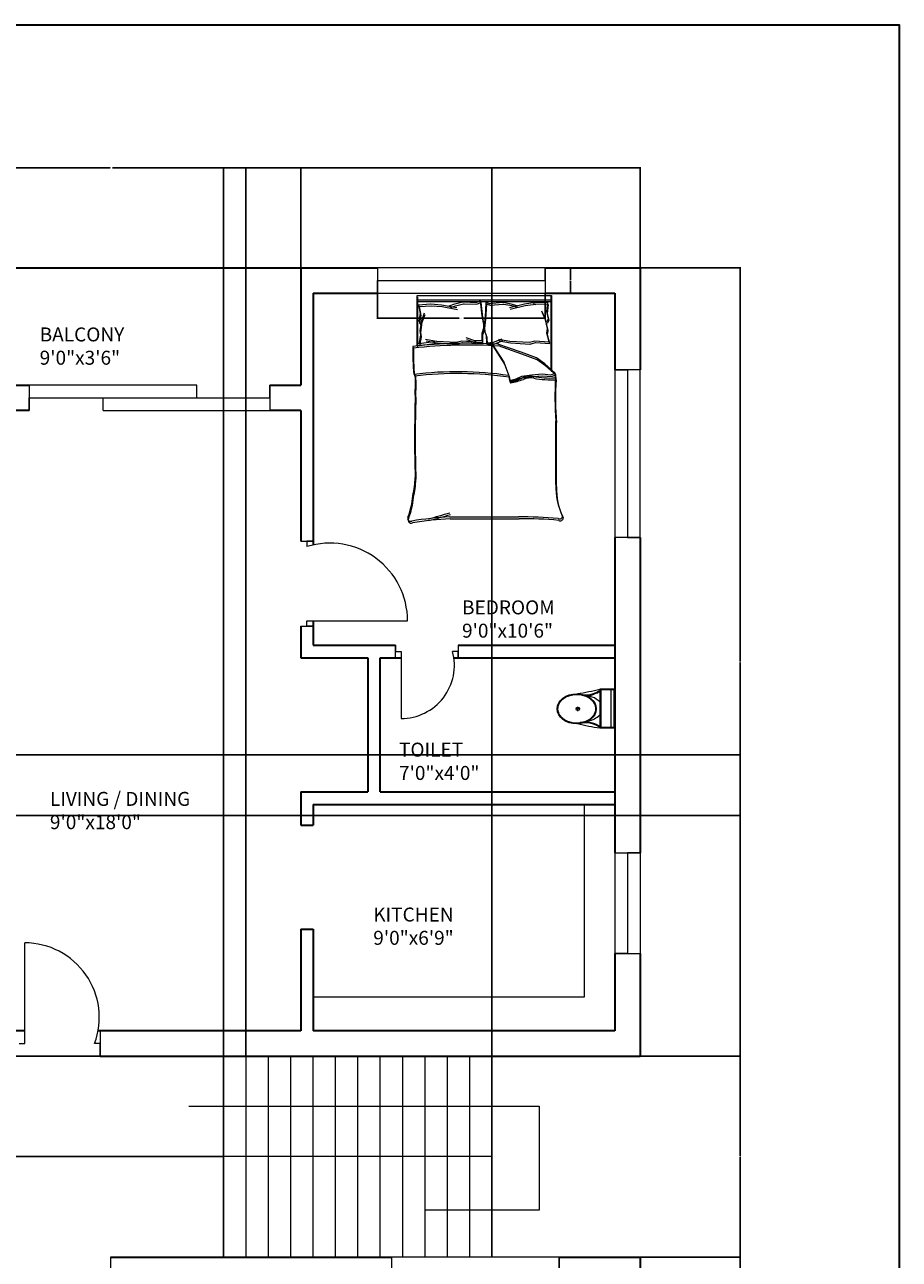
# Model space of a CAD drawing. Units: inches. Extents: x 2527 to 3140, y 1564 to 2435.
# Tile 4 of 4: x 2827 to 3140, y 1993 to 2435. Entities that reach past the tile are written whole.
import ezdxf

# ---------------------------------------------------------------- set-up
doc = ezdxf.new("R2010")
doc.units = ezdxf.units.IN
for name, color, linetype, lineweight in [('A-ANNO-DIMS', 2, 'Continuous', 18), ('A-ANNO-TTLB', 7, 'Continuous', 35), ('A-AREA-IDEN', 7, 'Continuous', 18), ('A-DOOR', 191, 'Continuous', 18), ('A-FLOR-CASE', 9, 'Continuous', 18), ('A-FLOR-FIXT', 7, 'Continuous', 18), ('A-FLOR-STRS', 81, 'Continuous', 18), ('A-FURN', 8, 'Continuous', 13), ('A-GLAZ', 131, 'Continuous', 18), ('A-WALL', 7, 'Continuous', 35)]:
    doc.layers.add(name, color=color, linetype=linetype, lineweight=lineweight)
doc.styles.get("Standard").update_dxf_attribs({"font": 'arial.ttf'})
doc.dimstyles.get("Standard").update_dxf_attribs({"dimtxt": 0.18, "dimasz": 0.18, "dimexe": 0.18, "dimexo": 0.0625, "dimgap": 0.09, "dimtad": 0, "dimtih": 1, "dimtoh": 1, "dimdec": 4, "dimzin": 0, "dimdsep": 46, "dimtxsty": 'Standard', "dimcen": 0.09, "dimadec": 0, "dimazin": 0, "dimtfac": 1, "dimtdec": 4, "dimtofl": 0, "dimtmove": 0, "dimatfit": 3, "dimfxl": 1, "dimtolj": 1, "dimtzin": 0, "dimarcsym": 0})

# ---------------------------------------------------------------- blocks, each defined once
blk = doc.blocks.new('A$C31115884')
for p, q in [((283, 498), (223, 498)), ((258, 466), (258, 523)), ((0, 200), (0, 0)), ((520, 200), (0, 200)), ((10, 190), (10, 10)), ((510, 190), (10, 190)), ((510, 10), (510, 190)), ((520, 0), (520, 200)), ((510, 54), (0, 54)), ((10, 10), (510, 10)), ((0, 0), (520, 0))]:
    blk.add_line(p, q)
blk.add_circle((256, 496), 23.6)
for centre, radius, start, end in [((2778, -205), 2807, 165.4549, 171.7133), ((3237, 905), 2807, 188.2867, 194.5451), ((-295, 403), 365, 324.2091, 9.3499), ((-295, 403), 375, 324.2091, 9.3499), ((384, 406), 293, 190.2774, 224.1564), ((139, 406), 293, 315.8436, 2.6563), ((806, 403), 375, 179.2036, 215.7909), ((806, 403), 365, 170.6501, 215.7909)]:
    blk.add_arc(centre, radius, start, end)
blk.add_ellipse((256, 510), major_axis=(0, -261), ratio=0.772727)
blk.add_open_spline([(256, 259), (263, 259), (270, 260), (288, 262), (299, 265), (320, 273), (330, 278), (350, 291), (360, 299), (378, 316), (386, 326), (402, 347), (409, 358), (421, 383), (427, 395), (436, 422), (440, 436), (445, 465), (447, 480), (448, 509), (448, 524), (445, 553), (443, 568), (436, 596), (432, 610), (422, 636), (416, 649), (402, 672), (395, 683), (379, 703), (370, 712), (351, 728), (341, 735), (321, 746), (310, 751), (289, 757), (278, 759), (256, 761), (245, 761), (223, 757), (212, 754), (191, 746), (181, 741), (161, 728), (151, 720), (133, 703), (125, 693), (110, 672), (103, 660), (90, 636), (85, 623), (76, 596), (72, 582), (67, 553), (66, 538), (64, 509), (65, 494), (68, 465), (70, 450), (77, 422), (81, 408), (91, 382), (97, 370), (111, 346), (118, 335), (135, 316), (144, 307), (162, 291), (172, 284), (193, 273), (203, 269), (225, 262), (236, 260), (250, 259), (253, 259), (256, 259)], degree=3, knots=[0, 0, 0, 0, 0.110105, 0.110105, 0.285049, 0.285049, 0.459994, 0.459994, 0.634938, 0.634938, 0.809882, 0.809882, 0.984827, 0.984827, 1.159771, 1.159771, 1.334715, 1.334715, 1.50966, 1.50966, 1.684604, 1.684604, 1.859549, 1.859549, 2.034493, 2.034493, 2.209437, 2.209437, 2.384382, 2.384382, 2.559326, 2.559326, 2.73427, 2.73427, 2.909215, 2.909215, 3.084159, 3.084159, 3.259103, 3.259103, 3.434048, 3.434048, 3.608992, 3.608992, 3.783936, 3.783936, 3.958881, 3.958881, 4.133825, 4.133825, 4.30877, 4.30877, 4.483714, 4.483714, 4.658658, 4.658658, 4.833603, 4.833603, 5.008547, 5.008547, 5.183491, 5.183491, 5.358436, 5.358436, 5.53338, 5.53338, 5.708324, 5.708324, 5.883269, 5.883269, 6.058213, 6.058213, 6.233158, 6.233158, 6.283185, 6.283185, 6.283185, 6.283185])
blk = doc.blocks.new('BED-DOUBLE')
for p, q in [((3.48, 63.33), (3.48, 81.44)), ((3.48, 63.33), (3.48, 81.44)), ((3.48, 81.44), (51.49, 81.44)), ((3.48, 79.91), (51.27, 79.91)), ((3.48, 79.91), (51.27, 79.91)), ((3.7, 62.69), (3.7, 80.8)), ((3.7, 62.69), (3.7, 80.8)), ((24.54, 78.99), (25.98, 79.57)), ((24.54, 78.99), (25.98, 79.57)), ((25.98, 79.57), (26.56, 74.22)), ((25.98, 79.57), (26.56, 74.22)), ((51.27, 81.44), (51.27, 54.83)), ((51.27, 81.44), (51.27, 54.83)), ((51.49, 81.44), (51.49, 80.8)), ((51.49, 80.8), (51.49, 54.19)), ((51.49, 80.8), (51.49, 54.19)), ((3.7, 79.27), (51.49, 79.27)), ((3.7, 79.27), (51.49, 79.27)), ((3.89, 78.13), (4.47, 74.95)), ((3.9, 78.1), (8.18, 78.43)), ((3.9, 78.1), (8.18, 78.43)), ((3.9, 78.13), (4.47, 74.95)), ((4.12, 77.49), (4.7, 74.31)), ((4.12, 77.49), (4.7, 74.31)), ((4.13, 77.47), (8.41, 77.79)), ((4.13, 77.47), (8.41, 77.79)), ((5.05, 72.49), (6.06, 75.24)), ((5.05, 72.49), (6.06, 75.24)), ((8.18, 78.43), (8.29, 78.42)), ((8.18, 78.43), (8.29, 78.42)), ((8.29, 78.42), (12.11, 78.13)), ((8.29, 78.42), (12.11, 78.13)), ((8.41, 77.79), (8.51, 77.78)), ((8.41, 77.79), (8.51, 77.78)), ((8.51, 77.78), (12.34, 77.49)), ((8.51, 77.78), (12.34, 77.49)), ((12.11, 78.13), (17.6, 77.11)), ((12.11, 78.13), (17.6, 77.11)), ((12.34, 77.49), (17.83, 76.48)), ((12.34, 77.49), (17.83, 76.48)), ((14.86, 77.69), (16.88, 78.42)), ((14.86, 77.69), (16.88, 78.42)), ((15.08, 77.05), (17.11, 77.78)), ((15.08, 77.05), (17.11, 77.78)), ((16.88, 78.42), (19.77, 79.14)), ((16.88, 78.42), (19.77, 79.14)), ((17.11, 77.78), (20, 78.5)), ((17.11, 77.78), (20, 78.5)), ((19.77, 79.14), (20.09, 79.14)), ((19.77, 79.14), (20.09, 79.14)), ((20, 78.5), (20.32, 78.5)), ((20, 78.5), (20.32, 78.5)), ((20.09, 79.14), (24.54, 78.99)), ((20.09, 79.14), (24.54, 78.99)), ((20.32, 78.5), (24.77, 78.35)), ((20.32, 78.5), (24.77, 78.35)), ((24.77, 78.35), (26.21, 78.93)), ((24.77, 78.35), (26.21, 78.93)), ((26.21, 78.93), (26.79, 73.58)), ((26.21, 78.93), (26.79, 73.58)), ((27.98, 78.95), (27.73, 73.58)), ((27.98, 78.95), (27.73, 73.58)), ((28.21, 78.31), (27.96, 72.94)), ((28.21, 78.31), (27.96, 72.94)), ((29.46, 78.46), (27.98, 78.95)), ((29.46, 78.46), (27.98, 78.95)), ((29.68, 77.82), (28.21, 78.31)), ((29.68, 77.82), (28.21, 78.31)), ((33.88, 78.89), (29.46, 78.46)), ((33.88, 78.89), (29.46, 78.46)), ((34.11, 78.25), (29.68, 77.82)), ((34.11, 78.25), (29.68, 77.82)), ((34.21, 78.91), (33.88, 78.89)), ((34.2, 78.91), (33.88, 78.89)), ((34.43, 78.27), (34.11, 78.25)), ((34.43, 78.27), (34.11, 78.25)), ((37.14, 78.36), (34.2, 78.91)), ((37.14, 78.36), (34.21, 78.91)), ((37.36, 77.73), (34.43, 78.27)), ((37.36, 77.73), (34.43, 78.27)), ((41.91, 78.37), (36.5, 77.02)), ((41.91, 78.37), (36.5, 77.02)), ((42.14, 77.73), (36.72, 76.38)), ((42.14, 77.73), (36.72, 76.38)), ((39.2, 77.77), (37.14, 78.36)), ((39.2, 77.77), (37.14, 78.36)), ((39.43, 77.13), (37.36, 77.73)), ((39.43, 77.13), (37.36, 77.73)), ((45.71, 78.9), (41.91, 78.37)), ((45.71, 78.9), (41.91, 78.37)), ((45.94, 78.26), (42.14, 77.73)), ((45.94, 78.26), (42.14, 77.73)), ((50.11, 78.89), (44.71, 78.98)), ((44.71, 78.98), (45.71, 78.9)), ((50.11, 78.89), (44.71, 78.98)), ((44.71, 78.98), (45.71, 78.9)), ((50.34, 78.25), (44.94, 78.34)), ((44.94, 78.34), (45.94, 78.26)), ((50.34, 78.25), (44.94, 78.34)), ((44.94, 78.34), (45.94, 78.26)), ((49.31, 73.19), (48.13, 75.86)), ((49.31, 73.19), (48.13, 75.86)), ((49.54, 72.55), (48.36, 75.23)), ((49.54, 72.55), (48.36, 75.23)), ((50.11, 78.89), (49.73, 75.68)), ((50.11, 78.89), (49.73, 75.68)), ((49.73, 75.68), (50.33, 73.1)), ((49.73, 75.68), (50.33, 73.1)), ((50.34, 78.25), (49.96, 75.04)), ((50.34, 78.25), (49.96, 75.04)), ((4.47, 74.95), (4.04, 72.34)), ((4.47, 74.95), (4.04, 72.34)), ((4.04, 72.34), (4.62, 71.33)), ((4.04, 72.34), (4.62, 71.33)), ((4.7, 74.31), (4.27, 71.7)), ((4.7, 74.31), (4.27, 71.7)), ((4.27, 71.7), (4.85, 70.69)), ((4.27, 71.7), (4.85, 70.69)), ((4.47, 68.87), (5.05, 72.49)), ((4.47, 68.87), (5.05, 72.49)), ((4.7, 68.23), (5.28, 71.85)), ((4.7, 68.23), (5.28, 71.85)), ((5.28, 71.85), (6.29, 74.6)), ((5.28, 71.85), (6.29, 74.6)), ((26.56, 74.22), (27.14, 71.04)), ((26.56, 74.22), (27.14, 71.04)), ((26.79, 73.58), (27.37, 70.4)), ((26.79, 73.58), (27.37, 70.4)), ((27.14, 71.04), (27.14, 69.74)), ((27.14, 71.04), (27.14, 69.74)), ((27.73, 73.58), (27.36, 70.36)), ((27.73, 73.58), (27.36, 70.36)), ((27.96, 72.94), (27.58, 69.73)), ((27.96, 72.94), (27.58, 69.73)), ((50.11, 69.61), (49.31, 73.19)), ((50.11, 69.61), (49.31, 73.19)), ((50.34, 68.97), (49.54, 72.55)), ((50.34, 68.97), (49.54, 72.55)), ((50.33, 73.1), (49.81, 72.06)), ((50.33, 73.1), (49.82, 72.06)), ((49.96, 75.04), (50.56, 72.47)), ((49.96, 75.04), (50.56, 72.47)), ((50.56, 72.47), (50.04, 71.42)), ((50.56, 72.47), (50.04, 71.42)), ((4.18, 64.1), (4.76, 67.28)), ((4.18, 64.1), (4.76, 67.28)), ((4.41, 63.46), (4.99, 66.64)), ((4.41, 63.46), (4.99, 66.64)), ((4.76, 67.28), (4.47, 68.87)), ((4.76, 67.28), (4.47, 68.87)), ((4.99, 66.64), (4.7, 68.23)), ((4.99, 66.64), (4.7, 68.23)), ((24.1, 65.18), (20.96, 66.27)), ((24.1, 65.18), (20.96, 66.27)), ((27.14, 69.74), (26.56, 67.86)), ((27.14, 69.74), (26.56, 67.86)), ((26.56, 67.86), (26.56, 65.18)), ((26.56, 67.86), (26.56, 65.18)), ((27.37, 69.1), (26.79, 67.22)), ((27.37, 69.1), (26.79, 67.22)), ((26.79, 67.22), (26.79, 64.54)), ((26.79, 67.22), (26.79, 64.54)), ((27.36, 70.36), (27.44, 69.07)), ((27.36, 70.36), (27.44, 69.07)), ((27.37, 70.4), (27.37, 69.1)), ((27.37, 70.4), (27.37, 69.1)), ((27.44, 69.07), (28.13, 67.23)), ((27.44, 69.07), (28.13, 67.23)), ((27.58, 69.73), (27.66, 68.43)), ((27.58, 69.73), (27.66, 68.43)), ((27.66, 68.43), (28.36, 66.59)), ((27.66, 68.43), (28.36, 66.59)), ((28.13, 67.23), (28.3, 64.55)), ((28.13, 67.23), (28.3, 64.55)), ((28.36, 66.59), (28.53, 63.91)), ((28.36, 66.59), (28.53, 63.91)), ((49.92, 68.01), (50.11, 69.61)), ((49.92, 68.01), (50.11, 69.61)), ((50.7, 64.87), (49.92, 68.01)), ((50.7, 64.87), (49.92, 68.01)), ((50.15, 67.37), (50.34, 68.97)), ((50.15, 67.37), (50.34, 68.97)), ((50.93, 64.23), (50.15, 67.37)), ((50.93, 64.23), (50.15, 67.37)), ((9.28, 64.82), (4.18, 64.1)), ((9.28, 64.82), (4.18, 64.1)), ((9.51, 64.19), (4.41, 63.46)), ((9.51, 64.19), (4.41, 63.46)), ((6.38, 65.81), (10.41, 65.15)), ((6.38, 65.81), (10.41, 65.15)), ((6.61, 65.17), (10.64, 64.51)), ((6.61, 65.17), (10.64, 64.51)), ((10.41, 65.15), (9.28, 64.82)), ((10.41, 65.15), (9.28, 64.82)), ((10.64, 64.51), (9.51, 64.19)), ((10.64, 64.51), (9.51, 64.19)), ((10.41, 65.15), (17.42, 64.72)), ((10.41, 65.15), (17.42, 64.72)), ((10.64, 64.51), (17.65, 64.08)), ((10.64, 64.51), (17.65, 64.08)), ((17.42, 64.72), (19.38, 65.27)), ((17.42, 64.72), (19.38, 65.27)), ((17.65, 64.08), (19.61, 64.63)), ((17.65, 64.08), (19.61, 64.63)), ((19.38, 65.27), (24.52, 64.87)), ((19.38, 65.27), (24.52, 64.87)), ((19.61, 64.63), (24.74, 64.23)), ((19.61, 64.63), (24.74, 64.23)), ((24.33, 64.54), (21.19, 65.63)), ((24.33, 64.54), (21.19, 65.63)), ((26.56, 65.18), (24.1, 65.18)), ((26.56, 65.18), (24.1, 65.18)), ((26.79, 64.54), (24.33, 64.54)), ((26.79, 64.54), (24.33, 64.54)), ((28.3, 64.55), (30.75, 64.7)), ((28.3, 64.55), (30.75, 64.7)), ((28.53, 63.91), (30.98, 64.06)), ((28.53, 63.91), (30.98, 64.06)), ((30.26, 64.06), (34.45, 57.57)), ((30.26, 64.06), (34.45, 57.57)), ((30.49, 63.42), (34.68, 56.93)), ((30.49, 63.42), (34.68, 56.93)), ((30.75, 64.7), (33.82, 65.99)), ((30.75, 64.7), (33.82, 65.99)), ((30.98, 64.06), (34.05, 65.35)), ((30.98, 64.06), (34.05, 65.35)), ((40.64, 61.13), (32.31, 64.06)), ((40.64, 61.13), (32.31, 64.06)), ((40.87, 60.49), (32.53, 63.42)), ((40.87, 60.49), (32.54, 63.42)), ((32.56, 65.81), (36.6, 65.15)), ((32.56, 65.81), (36.6, 65.15)), ((32.79, 65.17), (36.83, 64.51)), ((32.79, 65.17), (36.82, 64.51)), ((36.6, 65.15), (43.61, 64.72)), ((36.6, 65.15), (43.61, 64.72)), ((36.82, 64.51), (43.83, 64.08)), ((36.83, 64.51), (43.84, 64.08)), ((43.61, 64.72), (45.57, 65.27)), ((43.61, 64.72), (45.57, 65.27)), ((43.83, 64.08), (45.8, 64.63)), ((43.84, 64.08), (45.8, 64.63)), ((45.57, 65.27), (50.7, 64.87)), ((45.57, 65.27), (50.7, 64.87)), ((45.8, 64.63), (50.93, 64.23)), ((45.8, 64.63), (50.93, 64.23)), ((34.45, 57.57), (36.15, 53.08)), ((34.45, 57.57), (36.15, 53.08)), ((46.22, 59.11), (40.64, 61.13)), ((46.22, 59.11), (40.64, 61.13)), ((46.45, 58.47), (40.87, 60.49)), ((46.45, 58.47), (40.87, 60.49)), ((49.16, 56.95), (46.22, 59.11)), ((49.16, 56.95), (46.22, 59.11)), ((49.39, 56.31), (46.45, 58.47)), ((49.39, 56.31), (46.45, 58.47)), ((34.68, 56.93), (36.38, 52.44)), ((34.68, 56.93), (36.38, 52.44)), ((36.15, 53.08), (36.46, 51.07)), ((36.15, 53.08), (36.46, 51.07)), ((40.95, 52.61), (44.36, 53.08)), ((40.95, 52.61), (44.36, 53.08)), ((44.36, 53.08), (48.23, 53.39)), ((44.36, 53.08), (48.23, 53.39)), ((48.23, 53.39), (51.33, 53.08)), ((48.23, 53.39), (51.33, 53.08)), ((52.87, 53.7), (49.16, 56.95)), ((52.87, 53.7), (49.16, 56.95)), ((53.1, 53.06), (49.39, 56.31)), ((53.1, 53.06), (49.39, 56.31)), ((51.33, 53.08), (52.87, 53.7)), ((51.33, 53.08), (52.87, 53.7)), ((51.56, 52.44), (53.1, 53.06)), ((51.56, 52.44), (53.1, 53.06)), ((52.95, 51.95), (52.87, 53.7, 3.87)), ((52.95, 51.95), (52.87, 53.7, 3.87)), ((53.18, 51.31), (53.1, 53.06, 3.87)), ((53.18, 51.31), (53.1, 53.06, 3.87)), ((36.38, 52.44), (36.69, 50.43)), ((36.38, 52.44), (36.69, 50.43)), ((36.46, 51.07), (38.94, 51.68)), ((36.46, 51.07), (38.94, 51.68)), ((36.69, 50.43), (39.17, 51.05)), ((36.69, 50.43), (39.17, 51.05)), ((38.94, 51.68), (40.95, 52.61)), ((38.94, 51.68), (40.95, 52.61)), ((39.17, 51.05), (41.18, 51.97)), ((39.17, 51.05), (41.18, 51.97)), ((41.18, 51.97), (44.59, 52.44)), ((41.18, 51.97), (44.59, 52.44)), ((44.59, 52.44), (48.46, 52.75)), ((44.59, 52.44), (48.46, 52.75)), ((48.46, 52.75), (51.56, 52.44)), ((48.46, 52.75), (51.56, 52.44)), ((15.06, 2.2), (39.68, 2.2)), ((15.06, 2.2), (39.68, 2.2)), ((15.29, 1.56), (39.91, 1.56)), ((15.29, 1.56), (39.91, 1.56))]:
    blk.add_line(p, q)
for centre, radius, start, end in [((85.16, 61.35), 83.31, 178.7218, 185.604), ((85.16, 61.35), 83.31, 178.7218, 185.604), ((21.36, -100.61), 164.97, 86.0865, 96.7821), ((21.36, -100.61), 164.97, 86.0865, 96.7821), ((85.39, 60.71), 83.31, 178.7218, 185.604), ((85.39, 60.71), 83.31, 178.7218, 185.604), ((21.59, -101.25), 164.97, 86.0865, 96.7821), ((21.59, -101.25), 164.97, 86.0865, 96.7821), ((17.76, -74.87), 129.02, 81.7845, 96.9006), ((17.76, -74.87), 129.02, 81.7845, 96.9006), ((17.98, -75.51), 129.02, 81.7845, 96.9006), ((17.98, -75.51), 129.02, 81.7845, 96.9006), ((-167.31, 50.27), 170.11, 358.4762, 1.0082), ((-167.31, 50.27), 170.11, 358.4762, 1.0082), ((-167.08, 49.63), 170.11, 358.4762, 1.0082), ((-167.08, 49.63), 170.11, 358.4762, 1.0082), ((36.64, 51), 0.185, 160.2464, 271.1377), ((36.64, 51), 0.185, 160.2464, 271.1377), ((31.15, 79.96), 29.65, 280.6617, 289.8806), ((31.15, 79.96), 29.65, 280.6617, 289.8806), ((36.87, 50.36), 0.185, 160.2464, 271.1377), ((36.86, 50.36), 0.185, 160.2464, 271.1377), ((31.38, 79.32), 29.65, 280.6617, 289.8806), ((31.38, 79.32), 29.65, 280.6617, 289.8806), ((43.74, 46.38), 6.22, 78.6608, 113.7384), ((43.74, 46.38), 6.22, 78.6608, 113.7384), ((43.97, 45.74), 6.22, 78.6608, 113.7384), ((43.97, 45.74), 6.22, 78.6608, 113.7384), ((51.33, 88.1), 36.18, 259.8763, 272.5657), ((51.33, 88.1), 36.18, 259.8763, 272.5657), ((51.56, 87.46), 36.18, 259.8763, 272.5657), ((51.56, 87.46), 36.18, 259.8763, 272.5657), ((182.27, 45.13), 129.5, 176.9791, 183.8365), ((182.27, 45.13), 129.5, 176.9791, 183.8365), ((182.49, 44.49), 129.5, 176.9791, 183.8365), ((182.49, 44.49), 129.5, 176.9791, 183.8365), ((484.82, 30.83), 482.31, 178.2277, 181.7185), ((484.82, 30.83), 482.31, 178.2277, 181.7185), ((485.05, 30.19), 482.31, 178.2277, 181.7185), ((485.05, 30.19), 482.31, 178.2277, 181.7185), ((-4508.74, 13.62), 4561.86, 0.00217, 0.28689), ((-4508.74, 13.62), 4561.86, 0.00217, 0.28689), ((-4508.51, 12.98), 4561.86, 0.00217, 0.28689), ((-4508.51, 12.98), 4561.86, 0.00217, 0.28689), ((-26.9, 16.93), 29.63, 346.0648, 358.9113), ((-26.9, 16.93), 29.63, 346.0648, 358.9113), ((-26.67, 16.29), 29.63, 346.0648, 358.9113), ((-26.67, 16.29), 29.63, 346.0648, 358.9113), ((76.16, 12.78), 23.07, 177.4714, 206.4681), ((76.16, 12.78), 23.07, 177.4714, 206.4681), ((-21.66, 11.17), 23.56, 337.9751, 356.652), ((-21.66, 11.17), 23.56, 337.9751, 356.652), ((-21.43, 10.53), 23.56, 337.9751, 356.652), ((-21.43, 10.53), 23.56, 337.9751, 356.652), ((76.39, 12.14), 23.07, 177.4714, 206.4681), ((76.39, 12.14), 23.07, 177.4714, 206.4681), ((1.09, 1.73), 1.09, 146.1736, 293.4781), ((1.09, 1.73), 1.09, 146.1736, 293.4781), ((1.32, 1.09), 1.09, 146.1736, 293.4781), ((1.32, 1.09), 1.09, 146.1736, 293.4781), ((21.43, -119.39), 121.76, 92.9958, 99.4091), ((21.43, -119.39), 121.76, 92.9958, 99.4091), ((21.66, -120.03), 121.76, 92.9958, 99.4091), ((21.66, -120.03), 121.76, 92.9958, 99.4091), ((-17.22, 105.15), 106.46, 283.3832, 287.7053), ((-17.22, 105.15), 106.46, 283.3832, 287.7053), ((-16.99, 104.52), 106.46, 283.3832, 287.7053), ((-16.99, 104.52), 106.46, 283.3832, 287.7053), ((41.15, -130.83), 133.04, 84.4998, 90.6351), ((41.15, -130.83), 133.04, 84.4998, 90.6351), ((41.38, -131.47), 133.04, 84.4998, 90.6351), ((41.38, -131.47), 133.04, 84.4998, 90.6351), ((54.41, 2.57), 1.1, 242.6588, 356.02), ((54.41, 2.57), 1.1, 242.6588, 356.02), ((54.64, 1.93), 1.1, 242.6588, 356.02), ((54.64, 1.93), 1.1, 242.6588, 356.02)]:
    blk.add_arc(centre, radius, start, end)
blk = doc.blocks.new('WIN-60')
for p, q in [((0, 9), (0, 0)), ((60, 9), (0, 9)), ((60, 4.5), (60, 9)), ((60, 9), (60, 0)), ((0, 0), (0, 4.5)), ((0, 4.5), (60, 4.5)), ((0, 0), (60, 0))]:
    blk.add_line(p, q)
blk = doc.blocks.new('WIN-36')
for p, q in [((0, 36), (9, 36)), ((0, 36), (0, 0)), ((9, 36), (4.5, 36)), ((4.5, 36), (4.5, 0)), ((9, 36), (9, 0)), ((4.5, 0), (0, 0)), ((0, 0), (9, 0))]:
    blk.add_line(p, q)
blk = doc.blocks.new('*D7')
at = {"layer": 'A-ANNO-DIMS', "color": 0, "lineweight": -2, "transparency": 16777216}
for p, q in [((2953.62, 2339.08), (2953.62, 2329.96)), ((3013.62, 2339.08), (3013.62, 2329.96)), ((2953.8, 2330.14), (2982.77, 2330.14)), ((3013.44, 2330.14), (2984.46, 2330.14))]:
    blk.add_line(p, q, dxfattribs=at)
at = {"layer": 'A-ANNO-DIMS', "color": 0, "transparency": 16777216}
for points in [[(2953.8, 2330.17), (2953.8, 2330.11), (2953.62, 2330.14)], [(3013.44, 2330.17), (3013.44, 2330.11), (3013.62, 2330.14)]]:
    blk.add_solid(points, dxfattribs=at)
at = {"layer": 'Defpoints', "color": 0, "transparency": 16777216}
for p in [(2953.62, 2339.14), (3013.62, 2339.14), (3013.62, 2330.14)]:
    blk.add_point(p, dxfattribs=at)
at = {"layer": 'A-ANNO-DIMS', "color": 0, "transparency": 16777216, "insert": (2983.62, 2330.14), "char_height": 0.18, "attachment_point": 5}
blk.add_mtext('\\A1;WIN. 60 TYP.', dxfattribs=at)
blk = doc.blocks.new('*D8')
at = {"layer": 'A-ANNO-DIMS', "color": 0, "lineweight": -2, "transparency": 16777216}
for p, q in [((3013.68, 2348.14), (3022.8, 2348.14)), ((3022.62, 2347.96), (3022.62, 2343.82)), ((3022.62, 2339.32), (3022.62, 2343.46)), ((3013.68, 2339.14), (3022.8, 2339.14))]:
    blk.add_line(p, q, dxfattribs=at)
at = {"layer": 'A-ANNO-DIMS', "color": 0, "transparency": 16777216}
for points in [[(3022.59, 2347.96), (3022.65, 2347.96), (3022.62, 2348.14)], [(3022.59, 2339.32), (3022.65, 2339.32), (3022.62, 2339.14)]]:
    blk.add_solid(points, dxfattribs=at)
at = {"layer": 'Defpoints', "color": 0, "transparency": 16777216}
for p in [(3013.62, 2348.14), (3022.62, 2348.14), (3013.62, 2339.14)]:
    blk.add_point(p, dxfattribs=at)
at = {"layer": 'A-ANNO-DIMS', "color": 0, "transparency": 16777216, "insert": (3022.62, 2343.64), "char_height": 0.18, "attachment_point": 5}
blk.add_mtext('\\A1;9 TYP.', dxfattribs=at)
blk = doc.blocks.new('*D22')
at = {"layer": 'A-ANNO-DIMS', "color": 0, "lineweight": -2, "transparency": 16777216}
for p, q in [((2926.08, 2348.21), (2926.08, 2384.17)), ((2926.26, 2383.99), (2986.44, 2383.99)), ((3047.4, 2383.99), (2987.22, 2383.99)), ((3047.58, 2348.21), (3047.58, 2384.17))]:
    blk.add_line(p, q, dxfattribs=at)
at = {"layer": 'A-ANNO-DIMS', "color": 0, "transparency": 16777216}
for points in [[(2926.26, 2384.02), (2926.26, 2383.96), (2926.08, 2383.99)], [(3047.4, 2384.02), (3047.4, 2383.96), (3047.58, 2383.99)]]:
    blk.add_solid(points, dxfattribs=at)
at = {"layer": 'Defpoints', "color": 0, "transparency": 16777216}
for p in [(3047.58, 2383.99), (2926.08, 2348.14), (3047.58, 2348.14)]:
    blk.add_point(p, dxfattribs=at)
at = {"layer": 'A-ANNO-DIMS', "color": 0, "transparency": 16777216, "insert": (2986.83, 2383.99), "char_height": 0.18, "attachment_point": 5}
blk.add_mtext('\\A1;121.5', dxfattribs=at)
blk = doc.blocks.new('*D23')
at = {"layer": 'A-ANNO-DIMS', "color": 0, "lineweight": -2, "transparency": 16777216}
for p, q in [((3047.64, 1994.14), (3083.61, 1994.14)), ((3083.43, 1993.96), (3083.43, 1850.32)), ((3083.43, 1706.32), (3083.43, 1849.96)), ((3047.64, 1706.14), (3083.61, 1706.14))]:
    blk.add_line(p, q, dxfattribs=at)
at = {"layer": 'A-ANNO-DIMS', "color": 0, "transparency": 16777216}
for points in [[(3083.4, 1993.96), (3083.46, 1993.96), (3083.43, 1994.14)], [(3083.4, 1706.32), (3083.46, 1706.32), (3083.43, 1706.14)]]:
    blk.add_solid(points, dxfattribs=at)
at = {"layer": 'Defpoints', "color": 0, "transparency": 16777216}
for p in [(3047.58, 1994.14), (3083.43, 1994.14), (3047.58, 1706.14)]:
    blk.add_point(p, dxfattribs=at)
at = {"layer": 'A-ANNO-DIMS', "color": 0, "transparency": 16777216, "insert": (3083.43, 1850.14), "char_height": 0.18, "attachment_point": 5}
blk.add_mtext('\\A1;288', dxfattribs=at)
blk = doc.blocks.new('*D24')
at = {"layer": 'A-ANNO-DIMS', "color": 0, "lineweight": -2, "transparency": 16777216}
for p, q in [((3047.64, 2066.14), (3083.61, 2066.14)), ((3083.43, 2065.96), (3083.43, 2030.32)), ((3083.43, 1994.32), (3083.43, 2029.96)), ((3047.64, 1994.14), (3083.61, 1994.14))]:
    blk.add_line(p, q, dxfattribs=at)
at = {"layer": 'A-ANNO-DIMS', "color": 0, "transparency": 16777216}
for points in [[(3083.4, 2065.96), (3083.46, 2065.96), (3083.43, 2066.14)], [(3083.4, 1994.32), (3083.46, 1994.32), (3083.43, 1994.14)]]:
    blk.add_solid(points, dxfattribs=at)
at = {"layer": 'Defpoints', "color": 0, "transparency": 16777216}
for p in [(3047.58, 2066.14), (3083.43, 2066.14), (3047.58, 1994.14)]:
    blk.add_point(p, dxfattribs=at)
at = {"layer": 'A-ANNO-DIMS', "color": 0, "transparency": 16777216, "insert": (3083.43, 2030.14), "char_height": 0.18, "attachment_point": 5}
blk.add_mtext('\\A1;72', dxfattribs=at)
blk = doc.blocks.new('*D25')
at = {"layer": 'A-ANNO-DIMS', "color": 0, "lineweight": -2, "transparency": 16777216}
for p, q in [((3047.64, 2348.14), (3083.61, 2348.14)), ((3083.43, 2347.96), (3083.43, 2207.32)), ((3083.43, 2066.32), (3083.43, 2206.96)), ((3047.64, 2066.14), (3083.61, 2066.14))]:
    blk.add_line(p, q, dxfattribs=at)
at = {"layer": 'A-ANNO-DIMS', "color": 0, "transparency": 16777216}
for points in [[(3083.4, 2347.96), (3083.46, 2347.96), (3083.43, 2348.14)], [(3083.4, 2066.32), (3083.46, 2066.32), (3083.43, 2066.14)]]:
    blk.add_solid(points, dxfattribs=at)
at = {"layer": 'Defpoints', "color": 0, "transparency": 16777216}
for p in [(3047.58, 2348.14), (3083.43, 2348.14), (3047.58, 2066.14)]:
    blk.add_point(p, dxfattribs=at)
at = {"layer": 'A-ANNO-DIMS', "color": 0, "transparency": 16777216, "insert": (3083.43, 2207.14), "char_height": 0.18, "attachment_point": 5}
blk.add_mtext('\\A1;282', dxfattribs=at)
blk = doc.blocks.new('*D26')
at = {"layer": 'A-ANNO-DIMS', "color": 0, "lineweight": -2, "transparency": 16777216}
for p, q in [((2818.08, 1994.21), (2818.08, 2384.17)), ((2818.26, 2383.99), (2857.88, 2383.99)), ((2898.29, 2383.99), (2858.67, 2383.99)), ((2898.47, 1994.21), (2898.47, 2384.17))]:
    blk.add_line(p, q, dxfattribs=at)
at = {"layer": 'A-ANNO-DIMS', "color": 0, "transparency": 16777216}
for points in [[(2818.26, 2384.02), (2818.26, 2383.96), (2818.08, 2383.99)], [(2898.29, 2384.02), (2898.29, 2383.96), (2898.47, 2383.99)]]:
    blk.add_solid(points, dxfattribs=at)
at = {"layer": 'Defpoints', "color": 0, "transparency": 16777216}
for p in [(2898.47, 2383.99), (2818.08, 1994.14), (2898.47, 1994.14)]:
    blk.add_point(p, dxfattribs=at)
at = {"layer": 'A-ANNO-DIMS', "color": 0, "transparency": 16777216, "insert": (2858.27, 2383.99), "char_height": 0.18, "attachment_point": 5}
blk.add_mtext('\\A1;80.39', dxfattribs=at)
blk = doc.blocks.new('*D27')
at = {"layer": 'A-ANNO-DIMS', "color": 0, "lineweight": -2, "transparency": 16777216}
for p, q in [((2898.47, 1994.21), (2898.47, 2384.17)), ((2898.65, 2383.99), (2946.25, 2383.99)), ((2994.29, 2383.99), (2946.68, 2383.99)), ((2994.47, 1994.21), (2994.47, 2384.17))]:
    blk.add_line(p, q, dxfattribs=at)
at = {"layer": 'A-ANNO-DIMS', "color": 0, "transparency": 16777216}
for points in [[(2898.65, 2384.02), (2898.65, 2383.96), (2898.47, 2383.99)], [(2994.29, 2384.02), (2994.29, 2383.96), (2994.47, 2383.99)]]:
    blk.add_solid(points, dxfattribs=at)
at = {"layer": 'Defpoints', "color": 0, "transparency": 16777216}
for p in [(2994.47, 2383.99), (2898.47, 1994.14), (2994.47, 1994.14)]:
    blk.add_point(p, dxfattribs=at)
at = {"layer": 'A-ANNO-DIMS', "color": 0, "transparency": 16777216, "insert": (2946.47, 2383.99), "char_height": 0.18, "attachment_point": 5}
blk.add_mtext('\\A1;96', dxfattribs=at)
blk = doc.blocks.new('*D28')
at = {"layer": 'A-ANNO-DIMS', "color": 0, "lineweight": -2, "transparency": 16777216}
for p, q in [((2898.4, 2066.14), (2579.55, 2066.14)), ((2579.73, 2065.96), (2579.73, 2048.32)), ((2579.73, 2030.32), (2579.73, 2047.96)), ((2898.4, 2030.14), (2579.55, 2030.14))]:
    blk.add_line(p, q, dxfattribs=at)
at = {"layer": 'A-ANNO-DIMS', "color": 0, "transparency": 16777216}
for points in [[(2579.7, 2065.96), (2579.76, 2065.96), (2579.73, 2066.14)], [(2579.7, 2030.32), (2579.76, 2030.32), (2579.73, 2030.14)]]:
    blk.add_solid(points, dxfattribs=at)
at = {"layer": 'Defpoints', "color": 0, "transparency": 16777216}
for p in [(2579.73, 2066.14), (2898.47, 2066.14), (2898.47, 2030.14)]:
    blk.add_point(p, dxfattribs=at)
at = {"layer": 'A-ANNO-DIMS', "color": 0, "transparency": 16777216, "insert": (2579.73, 2048.14), "char_height": 0.18, "attachment_point": 5}
blk.add_mtext('\\A1;36', dxfattribs=at)
blk = doc.blocks.new('*D29')
at = {"layer": 'A-ANNO-DIMS', "color": 0, "lineweight": -2, "transparency": 16777216}
for p, q in [((2898.47, 2066.21), (2898.47, 2384.17)), ((2898.65, 2383.99), (2902.32, 2383.99)), ((2906.29, 2383.99), (2902.61, 2383.99)), ((2906.47, 2066.21), (2906.47, 2384.17))]:
    blk.add_line(p, q, dxfattribs=at)
at = {"layer": 'A-ANNO-DIMS', "color": 0, "transparency": 16777216}
for points in [[(2898.65, 2384.02), (2898.65, 2383.96), (2898.47, 2383.99)], [(2906.29, 2384.02), (2906.29, 2383.96), (2906.47, 2383.99)]]:
    blk.add_solid(points, dxfattribs=at)
at = {"layer": 'Defpoints', "color": 0, "transparency": 16777216}
for p in [(2906.47, 2383.99), (2898.47, 2066.14), (2906.47, 2066.14)]:
    blk.add_point(p, dxfattribs=at)
at = {"layer": 'A-ANNO-DIMS', "color": 0, "transparency": 16777216, "insert": (2902.47, 2383.99), "char_height": 0.18, "attachment_point": 5}
blk.add_mtext('\\A1;8', dxfattribs=at)
blk = doc.blocks.new('*D30')
at = {"layer": 'A-ANNO-DIMS', "color": 0, "lineweight": -2, "transparency": 16777216}
for p, q in [((2689.14, 2173.9), (3083.61, 2173.9)), ((3083.43, 2173.72), (3083.43, 2163.23)), ((3083.43, 2152.37), (3083.43, 2162.87)), ((2689.14, 2152.19), (3083.61, 2152.19))]:
    blk.add_line(p, q, dxfattribs=at)
at = {"layer": 'A-ANNO-DIMS', "color": 0, "transparency": 16777216}
for points in [[(3083.4, 2173.72), (3083.46, 2173.72), (3083.43, 2173.9)], [(3083.4, 2152.37), (3083.46, 2152.37), (3083.43, 2152.19)]]:
    blk.add_solid(points, dxfattribs=at)
at = {"layer": 'Defpoints', "color": 0, "transparency": 16777216}
for p in [(2689.08, 2173.9), (3083.43, 2173.9), (2689.08, 2152.19)]:
    blk.add_point(p, dxfattribs=at)
at = {"layer": 'A-ANNO-DIMS', "color": 0, "transparency": 16777216, "insert": (3083.43, 2163.05), "char_height": 0.18, "attachment_point": 5}
blk.add_mtext('\\A1;21.714', dxfattribs=at)

msp = doc.modelspace()

# ---------------------------------------------------------------- linework, layer by layer
at = {"layer": 'A-ANNO-TTLB'}
msp.add_lwpolyline([(2527.301, 2435.1781), (3140.3962, 2435.1781), (3140.3962, 1564.3652), (2527.301, 1564.3652)], close=True, dxfattribs=at)
at = {"layer": 'A-DOOR'}
for p, q in [((2828.8027, 2306.1426), (2828.8027, 2297.1426)), ((2888.8417, 2306.1426), (2828.8027, 2306.1426)), ((2888.8417, 2301.6426), (2888.8417, 2306.1426)), ((2915.0103, 2301.6426), (2915.0103, 2306.1426)), ((2915.0103, 2306.1426), (2915.0103, 2297.1426)), ((2828.8027, 2297.1426), (2828.8027, 2301.6426)), ((2828.8027, 2301.6426), (2915.0103, 2301.6426)), ((2855.3743, 2297.1426), (2855.3743, 2301.6426)), ((2855.3743, 2297.1426), (2915.0103, 2297.1426)), ((2926.0792, 2250.4041), (2930.5792, 2250.4041)), ((2930.5792, 2250.4041), (2928.3292, 2250.4041)), ((2928.3292, 2250.4041), (2928.3292, 2248.4041)), ((2926.0792, 2219.8926), (2930.5792, 2219.8926)), ((2928.3292, 2219.8926), (2928.3292, 2221.8926)), ((2928.3292, 2221.8926), (2964.3292, 2221.8926)), ((2930.5792, 2219.8926), (2928.3292, 2219.8926)), ((2960.0125, 2208.6426), (2960.0125, 2213.1426)), ((2960.0125, 2213.1426), (2960.0125, 2211.6736)), ((2960.0125, 2211.6736), (2960.0125, 2210.8926)), ((2960.0125, 2210.8926), (2962.0125, 2210.8926)), ((2962.0125, 2210.8926), (2962.0125, 2186.8926)), ((2982.461, 2210.8926), (2980.461, 2210.8926)), ((2982.461, 2213.1426), (2982.461, 2208.6426)), ((2982.461, 2208.6426), (2982.461, 2210.8926)), ((2827.2549, 2070.6426), (2827.2549, 2106.6426)), ((2854.305, 2075.1426), (2854.305, 2066.1426)), ((2825.2549, 2070.6426), (2827.2549, 2070.6426)), ((2854.305, 2070.6426), (2852.305, 2070.6426)), ((2854.305, 2066.1426), (2854.305, 2070.6426)), ((2857.9902, 1994.1426), (2857.9902, 1985.1426))]:
    msp.add_line(p, q, dxfattribs=at)
for centre, radius, start, end in [((2936.5672, 2221.8926), 27.762, 0, 107.261689), ((2962.0125, 2205.9832), 19.0906, 270, 14.901715), ((2827.2549, 2079.9272), 26.7154, 339.663223, 90)]:
    msp.add_arc(centre, radius, start, end, dxfattribs=at)
at = {"layer": 'A-FLOR-CASE'}
for p, q in [((3027.6473, 2087.2762), (3027.6473, 2156.1426)), ((2930.5792, 2087.2762), (3027.6473, 2087.2762))]:
    msp.add_line(p, q, dxfattribs=at)
at = {"layer": 'A-FLOR-STRS'}
for p, q in [((2898.4651, 2066.1426), (2898.4651, 1994.1426)), ((2906.4651, 2066.1426), (2906.4651, 1994.1426)), ((2914.4651, 2066.1426), (2914.4651, 1994.1426)), ((2922.4651, 2066.1426), (2922.4651, 1994.1426)), ((2930.4651, 2066.1426), (2930.4651, 1994.1426)), ((2938.4651, 2066.1426), (2938.4651, 1994.1426)), ((2946.4651, 2066.1426), (2946.4651, 1994.1426)), ((2954.4651, 2066.1426), (2954.4651, 1994.1426)), ((2962.4651, 2066.1426), (2962.4651, 1994.1426)), ((2970.4651, 2066.1426), (2970.4651, 1994.1426)), ((2978.4651, 2066.1426), (2978.4651, 1994.1426)), ((2986.4651, 2066.1426), (2986.4651, 1994.1426)), ((2994.4651, 2066.1426), (2994.4651, 1994.1426)), ((2886.0303, 2048.2292), (3011.4163, 2048.2292)), ((3011.4163, 2048.2292), (3011.4163, 2011.0114)), ((2994.4651, 2030.1426), (2898.4651, 2030.1426)), ((2994.4651, 1994.1426), (2994.4651, 2030.1426)), ((2994.4651, 2030.1426), (2994.4651, 2030.1426)), ((3011.4163, 2011.0114), (2970.4651, 2011.0114))]:
    msp.add_line(p, q, dxfattribs=at)
at = {"layer": 'A-WALL'}
for p, q in [((2818.0792, 2348.1426), (2926.0792, 2348.1426)), ((2926.0792, 2348.1426), (2926.0792, 2306.1426)), ((2926.0792, 2348.1426), (2953.6157, 2348.1426)), ((2926.0792, 2348.1426), (2953.6157, 2348.1426)), ((3013.6157, 2348.1426), (3047.5792, 2348.1426)), ((3013.6157, 2348.1426), (3047.5792, 2348.1426)), ((3047.5792, 2348.1426), (3047.5792, 2311.7191)), ((2930.5792, 2339.1426), (2930.5792, 2249.0011)), ((2930.5792, 2339.1426), (2953.6157, 2339.1426)), ((3013.6157, 2339.1426), (3038.5792, 2339.1426)), ((3038.5792, 2339.1426), (3038.5792, 2311.7191)), ((2818.0792, 2306.1426), (2828.8027, 2306.1426)), ((2915.0103, 2306.1426), (2926.0792, 2306.1426)), ((2828.8027, 2297.1426), (2818.0792, 2297.1426)), ((2926.0792, 2297.1426), (2915.0103, 2297.1426)), ((2926.0792, 2297.1426), (2926.0792, 2250.4041)), ((3038.5792, 2251.7191), (3038.5792, 2138.8158)), ((3047.5792, 2251.7191), (3047.5792, 2138.8158)), ((2926.0792, 2219.8926), (2926.0792, 2208.6426)), ((2930.5792, 2221.8926), (2930.5792, 2213.1426)), ((2930.5792, 2213.1426), (2960.0125, 2213.1426)), ((2982.461, 2213.1426), (3038.5792, 2213.1426)), ((2926.0792, 2208.6426), (2950.0792, 2208.6426)), ((2950.0792, 2208.6426), (2950.0792, 2160.6426)), ((2954.5792, 2160.6426), (2954.5792, 2208.6426)), ((2954.5792, 2208.6426), (2962.0125, 2208.6426)), ((2980.9169, 2208.6426), (3038.5792, 2208.6426)), ((2926.0792, 2160.6426), (2950.0792, 2160.6426)), ((2926.0792, 2160.6426), (2926.0792, 2148.7509)), ((2954.5792, 2160.6426), (3038.5792, 2160.6426)), ((2930.5792, 2156.1426), (3038.5792, 2156.1426)), ((2930.5792, 2156.1426), (2930.5792, 2148.7509)), ((3038.5792, 2156.1426), (3038.5792, 2138.8158)), ((2926.0792, 2148.7509), (2930.5792, 2148.7509)), ((2926.0792, 2111.5795), (2930.5792, 2111.5795)), ((2926.0792, 2111.5795), (2926.0792, 2075.1426)), ((2930.5792, 2111.5795), (2930.5792, 2075.1426)), ((3038.5792, 2102.8158), (3038.5792, 2075.1426)), ((3038.5792, 2102.8158), (3038.5792, 2075.1426)), ((3047.5792, 2102.8158), (3047.5792, 2066.1426)), ((2827.2549, 2075.1426), (2818.0792, 2075.1426)), ((2926.0792, 2075.1426), (2853.5383, 2075.1426)), ((3038.5792, 2075.1426), (2930.5792, 2075.1426)), ((2854.305, 2066.1426), (3047.5792, 2066.1426)), ((2857.9902, 1994.1426), (2958.601, 1994.1426)), ((3018.601, 1994.1426), (3047.5792, 1994.1426)), ((3047.5792, 1994.1426), (3047.5792, 1945.9238))]:
    msp.add_line(p, q, dxfattribs=at)

# ---------------------------------------------------------------- block references
at = {"layer": 'A-FLOR-FIXT', "xscale": 0.0268011493576733, "yscale": 0.0268011493576733, "zscale": 0.0268011493576733, "rotation": 90}
msp.add_blockref('A$C31115884', (3038.5792, 2183.5126), dxfattribs=at)
at = {"layer": 'A-FURN'}
msp.add_blockref('BED-DOUBLE', (2964.3354, 2256.8289), dxfattribs=at)
at = {"layer": 'A-GLAZ'}
for name, p in [('WIN-60', (2953.6161, 2339.143)), ('WIN-36', (3038.579, 2102.816)), ('WIN-60', (2958.6014, 1985.143))]:
    msp.add_blockref(name, p, dxfattribs=at)
at = {"layer": 'A-GLAZ', "rotation": 269.9999999999992}
msp.add_blockref('WIN-60', (3038.5796, 2311.7187), dxfattribs=at)

# ---------------------------------------------------------------- texts
at = {"layer": 'A-AREA-IDEN', "char_height": 5, "attachment_point": 1}
for s, width, insert in [('BALCONY\\P9\'0"x3\'6"', 116.135649, (2832.6199, 2326.8403)), ('BEDROOM\\P9\'0"x10\'6"', 121.252956, (2983.8353, 2229.1746)), ('TOILET\\P7\'0"x4\'0"', 83.469262, (2961.2746, 2178.2649)), ('LIVING / DINING \\P9\'0"x18\'0"', 101.790301, (2836.2889, 2160.6426)), ('KITCHEN\\P9\'0"x6\'9"', 129.524044, (2952.0567, 2119.2615))]:
    msp.add_mtext_dynamic_manual_height_columns(s, width=width, gutter_width=12.5, heights=[0], dxfattribs=dict(at, insert=insert))

# ---------------------------------------------------------------- dimensions: what is measured, and where the dimension line sits
at = {"layer": 'A-ANNO-DIMS'}
for base, p1, p2, override, picture, middle in [((2898.4651, 2383.9926), (2818.0792, 1994.1426), (2898.4651, 1994.1426), {"dimdec": 2, "dimlfac": 1, "dimrnd": 0, "dimzin": 0, "dimdsep": 46, "dimlunit": 2}, '*D26', (2858.2722, 2383.9926)), ((2994.4651, 2383.9926), (2898.4651, 1994.1426), (2994.4651, 1994.1426), {"dimdec": 0, "dimlfac": 1, "dimrnd": 0, "dimzin": 0, "dimdsep": 46, "dimlunit": 2}, '*D27', (2946.4651, 2383.9926)), ((2906.4651, 2383.9926), (2898.4651, 2066.1426), (2906.4651, 2066.1426), {"dimdec": 0, "dimlfac": 1, "dimrnd": 0, "dimzin": 0, "dimdsep": 46, "dimlunit": 2}, '*D29', (2902.4651, 2383.9926)), ((3047.5792, 2383.9926), (2926.0792, 2348.1426), (3047.5792, 2348.1426), {"dimdec": 1, "dimlfac": 1, "dimrnd": 0, "dimzin": 0, "dimdsep": 46, "dimlunit": 2}, '*D22', (2986.8292, 2383.9926))]:
    dim = msp.add_linear_dim(base=base, p1=p1, p2=p2, dimstyle='Standard', override=override, dxfattribs=at)
    dim.commit()
    dim.dimension.update_dxf_attribs({"geometry": picture, "text_midpoint": middle})
dim = msp.add_linear_dim(base=(3022.6157, 2348.1426), p1=(3013.6157, 2339.1426), p2=(3013.6157, 2348.1426), angle=90, text='<> TYP.', dimstyle='Standard', override={"dimdec": 0, "dimlfac": 1, "dimrnd": 0, "dimzin": 0, "dimdsep": 46, "dimlunit": 2}, dxfattribs=at)
dim.commit()
dim.dimension.update_dxf_attribs({"geometry": '*D8', "text_midpoint": (3022.6157, 2343.6426)})
for base, p1, p2, override, picture, middle in [((3083.4292, 2348.1426), (3047.5792, 2066.1426), (3047.5792, 2348.1426), {"dimdec": 0, "dimlfac": 1, "dimrnd": 0, "dimzin": 0, "dimdsep": 46, "dimlunit": 2}, '*D25', (3083.4292, 2207.1426)), ((3083.4292, 2173.9043), (2689.0792, 2152.1906), (2689.0792, 2173.9043), {"dimdec": 3, "dimlfac": 1, "dimrnd": 0, "dimzin": 0, "dimdsep": 46, "dimlunit": 2}, '*D30', (3083.4292, 2163.0474)), ((2579.7292, 2066.1426), (2898.4651, 2030.1426), (2898.4651, 2066.1426), {"dimdec": 0, "dimlfac": 1, "dimrnd": 0, "dimzin": 0, "dimdsep": 46, "dimlunit": 2}, '*D28', (2579.7292, 2048.1426)), ((3083.4292, 2066.1426), (3047.5792, 1994.1426), (3047.5792, 2066.1426), {"dimdec": 0, "dimlfac": 1, "dimrnd": 0, "dimzin": 0, "dimdsep": 46, "dimlunit": 2}, '*D24', (3083.4292, 2030.1426)), ((3083.4292, 1994.1426), (3047.5792, 1706.1426), (3047.5792, 1994.1426), {"dimdec": 0, "dimlfac": 1, "dimrnd": 0, "dimzin": 0, "dimdsep": 46, "dimlunit": 2}, '*D23', (3083.4292, 1850.1426))]:
    dim = msp.add_linear_dim(base=base, p1=p1, p2=p2, angle=90, dimstyle='Standard', override=override, dxfattribs=at)
    dim.commit()
    dim.dimension.update_dxf_attribs({"geometry": picture, "text_midpoint": middle})
dim = msp.add_linear_dim(base=(3013.6157, 2330.1426), p1=(2953.6157, 2339.1426), p2=(3013.6157, 2339.1426), text='WIN. <> TYP.', dimstyle='Standard', override={"dimdec": 0, "dimlfac": 1, "dimrnd": 0, "dimzin": 0, "dimdsep": 46, "dimlunit": 2}, dxfattribs=at)
dim.commit()
dim.dimension.update_dxf_attribs({"geometry": '*D7', "text_midpoint": (2983.6157, 2330.1426)})

doc.saveas('drawing.dxf')
